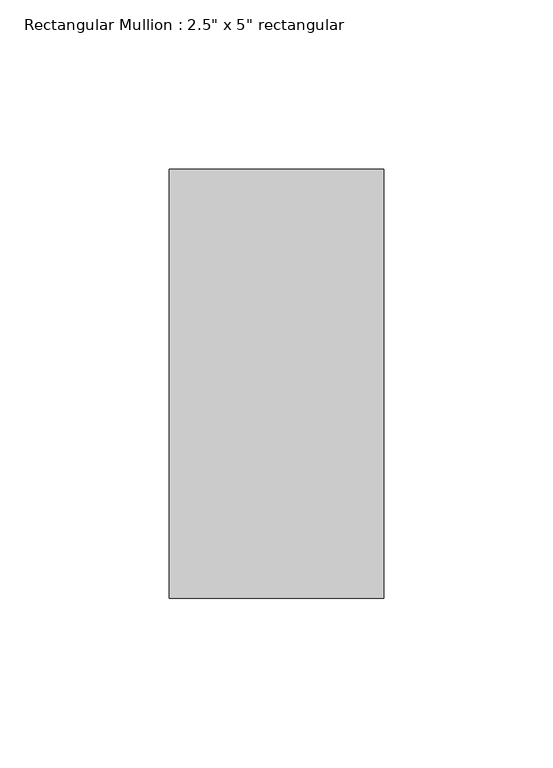
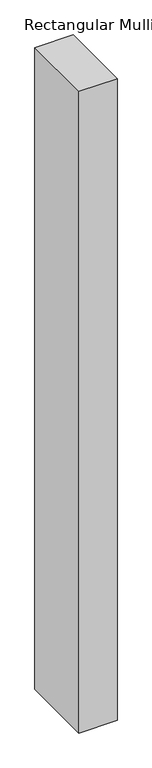
"""IFC4 building model written with IfcOpenShell, lengths in millimetres: member geometry."""

from ifc_helpers import new_model, si_unit, frame, origin, place, context, project, spatial, polyline, outline, extrude, source, transform, mapped, element, save


def member_fb055d8d(model_context):
    return source(origin(), model_context, "Body", "SweptSolid", [
        extrude(outline(polyline([(0.0, 63.5), (0.0, -63.5), (-63.5, -63.5), (-63.5, 63.5), (0.0, 63.5)])), frame((0.0, 0.0, -1130.2999998), z_axis=(0.0, 0.0, 1.0), x_axis=(1.0, 0.0, 0.0)), (0.0, 0.0, 1.0), 1130.2999998),
    ])


if __name__ == "__main__":
    model = new_model("IFC4")
    model_context = context("Model", 3, world=origin())
    ifc_project = project(units=[si_unit("LENGTHUNIT", "METRE", prefix="MILLI")], contexts=[model_context])
    site = spatial("IfcSite", under=ifc_project)
    building = spatial("IfcBuilding", under=site)
    placement = place(None, origin())
    member_shape = member_fb055d8d(model_context)
    element("IfcMember", 1, ObjectType="Rectangular Mullion : 2.5\" x 5\" rectangular", at=placement, inside=building, context=model_context, shape_type="MappedRepresentation", body=[
        mapped(member_shape, transform((0.0, 0.0, 0.0), x_axis=(1.0, 0.0, 0.0), y_axis=(0.0, 1.0, 0.0), z_axis=(0.0, 0.0, 1.0))),
    ])
    save(model, "model.ifc")

# Revit data of these elements
# Type "Rectangular Mullion : 2.5\" x 5\" rectangular"
#   built-in parameter 1007304 = 0.416667 (stored number, unit not read)
#   built-in parameter 1007301 = 0.104167 (stored number, unit not read)
#   built-in parameter 1007300 = 0.104167 (stored number, unit not read)
# Element 1 (IfcMember, "Rectangular Mullion : 2.5\" x 5\" rectangular")
#   Materials on its faces: "Aluminum"
# Materials
#   "Aluminum": class "Metal", colour RGB 247 247 247, transparency 0, Description = "Aluminum 6061", Cost = 0
